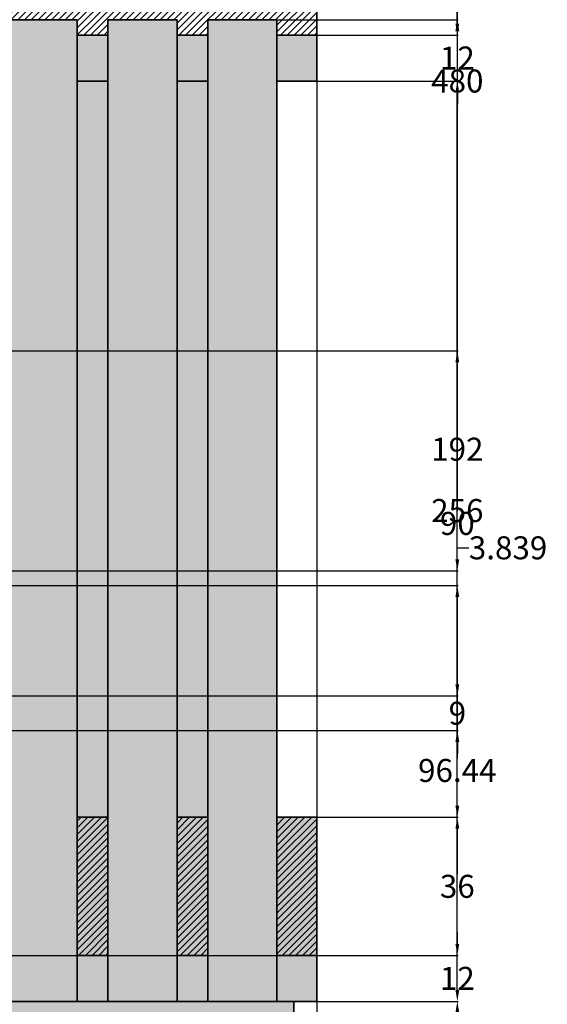
# Model space of a CAD drawing. Units: inches. Extents: x 126 to 726, y 86 to 888.
# Tile 11 of 13: x 589 to 726, y 354 to 611. Entities that reach past the tile are written whole.
import ezdxf

# ---------------------------------------------------------------- set-up
doc = ezdxf.new("R2010")
doc.units = ezdxf.units.IN
doc.header["$MEASUREMENT"] = 0
for name, color, linetype, lineweight in [('A-ANNO-DIMS', 2, 'Continuous', 18), ('A-ELEV', 7, 'Continuous', 35), ('A-ELEV-PATT', 8, 'Continuous', 13)]:
    doc.layers.add(name, color=color, linetype=linetype, lineweight=lineweight)
doc.styles.get("Standard").update_dxf_attribs({"font": 'arial.ttf'})
doc.dimstyles.get("Standard").update_dxf_attribs({"dimtxt": 6, "dimasz": 3, "dimexe": 0.18, "dimexo": 0.0625, "dimgap": 0.09, "dimtad": 0, "dimtih": 1, "dimtoh": 1, "dimdec": 0, "dimzin": 0, "dimdsep": 46, "dimlunit": 3, "dimtxsty": 'Standard', "dimcen": 0.09, "dimadec": 0, "dimazin": 0, "dimtfac": 1, "dimtdec": 0, "dimtofl": 0, "dimtmove": 0, "dimatfit": 3, "dimfxl": 1, "dimtolj": 1, "dimtzin": 0, "dimarcsym": 0})

# ---------------------------------------------------------------- blocks, each defined once
blk = doc.blocks.new('*D13')
at = {"layer": 'A-ANNO-DIMS', "color": 0, "lineweight": -2, "transparency": 16777216}
for p, q in [((665.97, 642.98), (665.97, 90.21)), ((185.97, 126.98), (185.97, 90.21)), ((188.97, 90.39), (419.15, 90.39)), ((662.97, 90.39), (432.8, 90.39))]:
    blk.add_line(p, q, dxfattribs=at)
at = {"layer": 'A-ANNO-DIMS', "color": 0, "transparency": 16777216}
for points in [[(188.97, 90.89), (188.97, 89.89), (185.97, 90.39)], [(662.97, 90.89), (662.97, 89.89), (665.97, 90.39)]]:
    blk.add_solid(points, dxfattribs=at)
at = {"layer": 'Defpoints', "color": 0, "transparency": 16777216}
for p in [(665.97, 643.04), (185.97, 127.04), (665.97, 90.39)]:
    blk.add_point(p, dxfattribs=at)
at = {"layer": 'A-ANNO-DIMS', "color": 0, "transparency": 16777216, "insert": (425.97, 90.39), "char_height": 6, "attachment_point": 5}
blk.add_mtext('\\A1;480', dxfattribs=at)
blk = doc.blocks.new('*D28')
at = {"layer": 'A-ANNO-DIMS', "color": 0, "lineweight": -2, "transparency": 16777216}
for p, q in [((666.04, 355.04), (702.8, 355.04)), ((702.62, 352.04), (702.62, 244.2)), ((702.62, 130.04), (702.62, 237.89)), ((660.11, 127.04), (702.8, 127.04))]:
    blk.add_line(p, q, dxfattribs=at)
at = {"layer": 'A-ANNO-DIMS', "color": 0, "transparency": 16777216}
for points in [[(702.12, 352.04), (703.12, 352.04), (702.62, 355.04)], [(702.12, 130.04), (703.12, 130.04), (702.62, 127.04)]]:
    blk.add_solid(points, dxfattribs=at)
at = {"layer": 'Defpoints', "color": 0, "transparency": 16777216}
for p in [(665.97, 355.04), (702.62, 355.04), (660.05, 127.04)]:
    blk.add_point(p, dxfattribs=at)
at = {"layer": 'A-ANNO-DIMS', "color": 0, "transparency": 16777216, "insert": (702.62, 241.04), "char_height": 6, "attachment_point": 5}
blk.add_mtext('\\A1;228', dxfattribs=at)
blk = doc.blocks.new('*D29')
at = {"layer": 'A-ANNO-DIMS', "color": 0, "lineweight": -2, "transparency": 16777216}
for p, q in [((606.04, 835.04), (702.8, 835.04)), ((702.62, 832.04), (702.62, 598.2)), ((702.62, 358.04), (702.62, 591.89)), ((666.04, 355.04), (702.8, 355.04))]:
    blk.add_line(p, q, dxfattribs=at)
at = {"layer": 'A-ANNO-DIMS', "color": 0, "transparency": 16777216}
for points in [[(702.12, 832.04), (703.12, 832.04), (702.62, 835.04)], [(702.12, 358.04), (703.12, 358.04), (702.62, 355.04)]]:
    blk.add_solid(points, dxfattribs=at)
at = {"layer": 'Defpoints', "color": 0, "transparency": 16777216}
for p in [(605.97, 835.04), (702.62, 835.04), (665.97, 355.04)]:
    blk.add_point(p, dxfattribs=at)
at = {"layer": 'A-ANNO-DIMS', "color": 0, "transparency": 16777216, "insert": (702.62, 595.04), "char_height": 6, "attachment_point": 5}
blk.add_mtext('\\A1;480', dxfattribs=at)
blk = doc.blocks.new('*D34')
at = {"layer": 'A-ANNO-DIMS', "color": 0, "lineweight": -2, "transparency": 16777216}
for p, q in [((362.73, 524.68), (702.8, 524.68)), ((702.62, 521.68), (702.62, 482.84)), ((702.62, 437.68), (702.62, 476.53)), ((362.73, 434.68), (702.8, 434.68))]:
    blk.add_line(p, q, dxfattribs=at)
at = {"layer": 'A-ANNO-DIMS', "color": 0, "transparency": 16777216}
for points in [[(702.12, 521.68), (703.12, 521.68), (702.62, 524.68)], [(702.12, 437.68), (703.12, 437.68), (702.62, 434.68)]]:
    blk.add_solid(points, dxfattribs=at)
at = {"layer": 'Defpoints', "color": 0, "transparency": 16777216}
for p in [(362.67, 524.68), (702.62, 524.68), (362.67, 434.68)]:
    blk.add_point(p, dxfattribs=at)
at = {"layer": 'A-ANNO-DIMS', "color": 0, "transparency": 16777216, "insert": (702.62, 479.68), "char_height": 6, "attachment_point": 5}
blk.add_mtext('\\A1;90', dxfattribs=at)
blk = doc.blocks.new('*D35')
at = {"layer": 'A-ANNO-DIMS', "color": 0, "lineweight": -2, "transparency": 16777216}
for p, q in [((702.624909, 437.684516), (702.624909, 440.684516)), ((362.728342, 434.684516), (702.804909, 434.684516)), ((371.728342, 425.684516), (702.804909, 425.684516)), ((702.624909, 422.684516), (702.624909, 419.684516))]:
    blk.add_line(p, q, dxfattribs=at)
at = {"layer": 'A-ANNO-DIMS', "color": 0, "transparency": 16777216}
for points in [[(702.124909, 437.684516), (703.124909, 437.684516), (702.624909, 434.684516)], [(702.124909, 422.684516), (703.124909, 422.684516), (702.624909, 425.684516)]]:
    blk.add_solid(points, dxfattribs=at)
at = {"layer": 'Defpoints', "color": 0, "transparency": 16777216}
for p in [(362.665842, 434.684516), (702.624909, 434.684516), (371.665842, 425.684516)]:
    blk.add_point(p, dxfattribs=at)
at = {"layer": 'A-ANNO-DIMS', "color": 0, "transparency": 16777216, "insert": (702.624909, 430.184516), "char_height": 6, "attachment_point": 5}
blk.add_mtext('\\A1;9', dxfattribs=at)
blk = doc.blocks.new('*D41')
at = {"layer": 'A-ANNO-DIMS', "color": 0, "lineweight": -2, "transparency": 16777216}
for p, q in [((429.97, 607.1), (429.97, 883.87)), ((432.97, 883.69), (541.21, 883.69)), ((662.97, 883.69), (554.74, 883.69)), ((665.97, 607.1), (665.97, 883.87))]:
    blk.add_line(p, q, dxfattribs=at)
at = {"layer": 'A-ANNO-DIMS', "color": 0, "transparency": 16777216}
for points in [[(432.97, 884.19), (432.97, 883.19), (429.97, 883.69)], [(662.97, 884.19), (662.97, 883.19), (665.97, 883.69)]]:
    blk.add_solid(points, dxfattribs=at)
at = {"layer": 'Defpoints', "color": 0, "transparency": 16777216}
for p in [(665.97, 883.69), (429.97, 607.04), (665.97, 607.04)]:
    blk.add_point(p, dxfattribs=at)
at = {"layer": 'A-ANNO-DIMS', "color": 0, "transparency": 16777216, "insert": (547.97, 883.69), "char_height": 6, "attachment_point": 5}
blk.add_mtext('\\A1;236', dxfattribs=at)
blk = doc.blocks.new('*D42')
at = {"layer": 'A-ANNO-DIMS', "color": 0, "lineweight": -2, "transparency": 16777216}
for p, q in [((429.97, 354.98), (429.97, 90.21)), ((665.97, 354.98), (665.97, 90.21)), ((432.97, 90.39), (541.21, 90.39)), ((662.97, 90.39), (554.74, 90.39))]:
    blk.add_line(p, q, dxfattribs=at)
at = {"layer": 'A-ANNO-DIMS', "color": 0, "transparency": 16777216}
for points in [[(432.97, 90.89), (432.97, 89.89), (429.97, 90.39)], [(662.97, 90.89), (662.97, 89.89), (665.97, 90.39)]]:
    blk.add_solid(points, dxfattribs=at)
at = {"layer": 'Defpoints', "color": 0, "transparency": 16777216}
for p in [(429.97, 355.04), (665.97, 355.04), (665.97, 90.39)]:
    blk.add_point(p, dxfattribs=at)
at = {"layer": 'A-ANNO-DIMS', "color": 0, "transparency": 16777216, "insert": (547.97, 90.39), "char_height": 6, "attachment_point": 5}
blk.add_mtext('\\A1;236', dxfattribs=at)
blk = doc.blocks.new('*D45')
at = {"layer": 'A-ANNO-DIMS', "color": 0, "lineweight": -2, "transparency": 16777216}
for p, q in [((702.624909, 370.042369), (702.624909, 373.042369)), ((666.037409, 367.042369), (702.804909, 367.042369)), ((666.037409, 355.042369), (702.804909, 355.042369)), ((702.624909, 352.042369), (702.624909, 349.042369))]:
    blk.add_line(p, q, dxfattribs=at)
at = {"layer": 'A-ANNO-DIMS', "color": 0, "transparency": 16777216}
for points in [[(702.124909, 370.042369), (703.124909, 370.042369), (702.624909, 367.042369)], [(702.124909, 352.042369), (703.124909, 352.042369), (702.624909, 355.042369)]]:
    blk.add_solid(points, dxfattribs=at)
at = {"layer": 'Defpoints', "color": 0, "transparency": 16777216}
for p in [(665.974909, 367.042369), (702.624909, 367.042369), (665.974909, 355.042369)]:
    blk.add_point(p, dxfattribs=at)
at = {"layer": 'A-ANNO-DIMS', "color": 0, "transparency": 16777216, "insert": (702.624909, 361.042369), "char_height": 6, "attachment_point": 5}
blk.add_mtext('\\A1;12', dxfattribs=at)
blk = doc.blocks.new('*D46')
at = {"layer": 'A-ANNO-DIMS', "color": 0, "lineweight": -2, "transparency": 16777216}
for p, q in [((666.04, 403.04), (702.8, 403.04)), ((702.62, 400.04), (702.62, 388.2)), ((702.62, 370.04), (702.62, 381.89)), ((666.04, 367.04), (702.8, 367.04))]:
    blk.add_line(p, q, dxfattribs=at)
at = {"layer": 'A-ANNO-DIMS', "color": 0, "transparency": 16777216}
for points in [[(702.12, 400.04), (703.12, 400.04), (702.62, 403.04)], [(702.12, 370.04), (703.12, 370.04), (702.62, 367.04)]]:
    blk.add_solid(points, dxfattribs=at)
at = {"layer": 'Defpoints', "color": 0, "transparency": 16777216}
for p in [(665.97, 403.04), (702.62, 403.04), (665.97, 367.04)]:
    blk.add_point(p, dxfattribs=at)
at = {"layer": 'A-ANNO-DIMS', "color": 0, "transparency": 16777216, "insert": (702.62, 385.04), "char_height": 6, "attachment_point": 5}
blk.add_mtext('\\A1;36', dxfattribs=at)
blk = doc.blocks.new('*D47')
at = {"layer": 'A-ANNO-DIMS', "color": 0, "lineweight": -2, "transparency": 16777216}
for p, q in [((666.04, 595.04), (702.8, 595.04)), ((702.62, 592.04), (702.62, 502.2)), ((702.62, 406.04), (702.62, 495.89)), ((666.04, 403.04), (702.8, 403.04))]:
    blk.add_line(p, q, dxfattribs=at)
at = {"layer": 'A-ANNO-DIMS', "color": 0, "transparency": 16777216}
for points in [[(702.12, 592.04), (703.12, 592.04), (702.62, 595.04)], [(702.12, 406.04), (703.12, 406.04), (702.62, 403.04)]]:
    blk.add_solid(points, dxfattribs=at)
at = {"layer": 'Defpoints', "color": 0, "transparency": 16777216}
for p in [(665.97, 595.04), (702.62, 595.04), (665.97, 403.04)]:
    blk.add_point(p, dxfattribs=at)
at = {"layer": 'A-ANNO-DIMS', "color": 0, "transparency": 16777216, "insert": (702.62, 499.04), "char_height": 6, "attachment_point": 5}
blk.add_mtext('\\A1;192', dxfattribs=at)
blk = doc.blocks.new('*D48')
at = {"layer": 'A-ANNO-DIMS', "color": 0, "lineweight": -2, "transparency": 16777216}
for p, q in [((702.624909, 610.042369), (702.624909, 613.042369)), ((666.037409, 607.042369), (702.804909, 607.042369)), ((666.037409, 595.042369), (702.804909, 595.042369)), ((702.624909, 592.042369), (702.624909, 589.042369))]:
    blk.add_line(p, q, dxfattribs=at)
at = {"layer": 'A-ANNO-DIMS', "color": 0, "transparency": 16777216}
for points in [[(702.124909, 610.042369), (703.124909, 610.042369), (702.624909, 607.042369)], [(702.124909, 592.042369), (703.124909, 592.042369), (702.624909, 595.042369)]]:
    blk.add_solid(points, dxfattribs=at)
at = {"layer": 'Defpoints', "color": 0, "transparency": 16777216}
for p in [(665.974909, 607.042369), (702.624909, 607.042369), (665.974909, 595.042369)]:
    blk.add_point(p, dxfattribs=at)
at = {"layer": 'A-ANNO-DIMS', "color": 0, "transparency": 16777216, "insert": (702.624909, 601.042369), "char_height": 6, "attachment_point": 5}
blk.add_mtext('\\A1;12', dxfattribs=at)
blk = doc.blocks.new('*D49')
at = {"layer": 'A-ANNO-DIMS', "color": 0, "lineweight": -2, "transparency": 16777216}
for p, q in [((666.04, 643.04), (702.8, 643.04)), ((702.62, 640.04), (702.62, 628.2)), ((702.62, 610.04), (702.62, 621.89)), ((666.04, 607.04), (702.8, 607.04))]:
    blk.add_line(p, q, dxfattribs=at)
at = {"layer": 'A-ANNO-DIMS', "color": 0, "transparency": 16777216}
for points in [[(702.12, 640.04), (703.12, 640.04), (702.62, 643.04)], [(702.12, 610.04), (703.12, 610.04), (702.62, 607.04)]]:
    blk.add_solid(points, dxfattribs=at)
at = {"layer": 'Defpoints', "color": 0, "transparency": 16777216}
for p in [(665.97, 643.04), (702.62, 643.04), (665.97, 607.04)]:
    blk.add_point(p, dxfattribs=at)
at = {"layer": 'A-ANNO-DIMS', "color": 0, "transparency": 16777216, "insert": (702.62, 625.04), "char_height": 6, "attachment_point": 5}
blk.add_mtext('\\A1;36', dxfattribs=at)
blk = doc.blocks.new('*D57')
at = {"layer": 'A-ANNO-DIMS', "color": 0, "lineweight": -2, "transparency": 16777216}
for p, q in [((655.64, 611.04), (702.8, 611.04)), ((702.62, 608.04), (702.62, 486.2)), ((702.62, 358.04), (702.62, 479.89)), ((655.64, 355.04), (702.8, 355.04))]:
    blk.add_line(p, q, dxfattribs=at)
at = {"layer": 'A-ANNO-DIMS', "color": 0, "transparency": 16777216}
for points in [[(702.12, 608.04), (703.12, 608.04), (702.62, 611.04)], [(702.12, 358.04), (703.12, 358.04), (702.62, 355.04)]]:
    blk.add_solid(points, dxfattribs=at)
at = {"layer": 'Defpoints', "color": 0, "transparency": 16777216}
for p in [(655.58, 611.04), (702.62, 611.04), (655.58, 355.04)]:
    blk.add_point(p, dxfattribs=at)
at = {"layer": 'A-ANNO-DIMS', "color": 0, "transparency": 16777216, "insert": (702.62, 483.04), "char_height": 6, "attachment_point": 5}
blk.add_mtext('\\A1;256', dxfattribs=at)
blk = doc.blocks.new('*D62')
at = {"layer": 'A-ANNO-DIMS', "color": 0, "lineweight": -2, "transparency": 16777216}
for p, q in [((702.62, 470.32), (702.62, 473.32)), ((702.62, 473.32), (705.62, 473.32)), ((515.5, 467.32), (702.8, 467.32)), ((515.5, 463.48), (702.8, 463.48)), ((702.62, 460.48), (702.62, 457.48))]:
    blk.add_line(p, q, dxfattribs=at)
at = {"layer": 'A-ANNO-DIMS', "color": 0, "transparency": 16777216}
for points in [[(702.12, 470.32), (703.12, 470.32), (702.62, 467.32)], [(702.12, 460.48), (703.12, 460.48), (702.62, 463.48)]]:
    blk.add_solid(points, dxfattribs=at)
at = {"layer": 'Defpoints', "color": 0, "transparency": 16777216}
for p in [(515.44, 467.32), (702.62, 467.32), (515.44, 463.48)]:
    blk.add_point(p, dxfattribs=at)
at = {"layer": 'A-ANNO-DIMS', "color": 0, "transparency": 16777216, "insert": (715.84, 473.32), "char_height": 6, "attachment_point": 5}
blk.add_mtext('\\A1;3.839', dxfattribs=at)
blk = doc.blocks.new('*D64')
at = {"layer": 'A-ANNO-DIMS', "color": 0, "lineweight": -2, "transparency": 16777216}
for p, q in [((501.88, 463.48), (702.8, 463.48)), ((702.62, 460.48), (702.62, 418.42)), ((702.62, 370.04), (702.62, 412.11)), ((486.04, 367.04), (702.8, 367.04))]:
    blk.add_line(p, q, dxfattribs=at)
at = {"layer": 'A-ANNO-DIMS', "color": 0, "transparency": 16777216}
for points in [[(702.12, 460.48), (703.12, 460.48), (702.62, 463.48)], [(702.12, 370.04), (703.12, 370.04), (702.62, 367.04)]]:
    blk.add_solid(points, dxfattribs=at)
at = {"layer": 'Defpoints', "color": 0, "transparency": 16777216}
for p in [(501.82, 463.48), (485.97, 367.04), (702.62, 367.04)]:
    blk.add_point(p, dxfattribs=at)
at = {"layer": 'A-ANNO-DIMS', "color": 0, "transparency": 16777216, "insert": (702.62, 415.26), "char_height": 6, "attachment_point": 5}
blk.add_mtext('\\A1;96.44', dxfattribs=at)

msp = doc.modelspace()

# ---------------------------------------------------------------- hatches: boundary and pattern name
at = {"layer": 'A-ELEV-PATT'}
h = msp.add_hatch(dxfattribs=at)
h.set_pattern_fill('ANSI31', color=256, scale=10)
h.paths.add_polyline_path([(585.5818, 607.0424), (585.5818, 611.0424), (603.5818, 611.0424), (603.5818, 607.0424), (611.5818, 607.0424), (611.5818, 611.0424), (629.5818, 611.0424), (629.5818, 607.0424), (637.5818, 607.0424), (637.5818, 611.0424), (655.5818, 611.0424), (655.5818, 607.0424), (665.9749, 607.0424), (665.9749, 643.0424), (485.9749, 643.0424), (485.9749, 607.0424)])
h = msp.add_hatch(color=256, dxfattribs=at)
h.dxf.hatch_style = 1
h.paths.add_polyline_path([(655.5818, 607.0424), (655.5818, 611.0424), (637.5818, 611.0424), (637.5818, 355.0424), (655.5818, 355.0424)])
h.paths.add_polyline_path([(629.5818, 611.0424), (611.5818, 611.0424), (611.5818, 355.0424), (629.5818, 355.0424)])
h.paths.add_polyline_path([(585.5818, 355.0424), (603.5818, 355.0424), (603.5818, 611.0424), (585.5818, 611.0424), (585.5818, 607.0424)])
h = msp.add_hatch(color=256, dxfattribs=at)
h.dxf.hatch_style = 1
h.paths.add_polyline_path([(611.5818, 367.0424), (603.5818, 367.0424), (603.5818, 355.0424), (611.5818, 355.0424)])
h.paths.add_polyline_path([(637.5818, 355.0424), (637.5818, 367.0424), (629.5818, 367.0424), (629.5818, 355.0424)])
h.paths.add_polyline_path([(665.9749, 355.0424), (665.9749, 367.0424), (655.5818, 367.0424), (655.5818, 355.0424)])
h.paths.add_polyline_path([(665.9749, 607.0424), (655.5818, 607.0424), (655.5818, 595.0424), (665.9749, 595.0424)])
h.paths.add_polyline_path([(629.5818, 595.0424), (637.5818, 595.0424), (637.5818, 607.0424), (629.5818, 607.0424)])
h.paths.add_polyline_path([(603.5818, 595.0424), (611.5818, 595.0424), (611.5818, 607.0424), (603.5818, 607.0424)])
h = msp.add_hatch(color=256, dxfattribs=at)
h.dxf.hatch_style = 1
h.paths.add_polyline_path([(485.9749, 595.0424), (485.9749, 564.6845), (585.5818, 564.6845), (585.5818, 595.0424)])
h.paths.add_polyline_path([(660.0469, 325.0424), (660.0469, 355.0424), (485.9749, 355.0424), (485.9749, 325.0424)])
h = msp.add_hatch(color=256, dxfattribs=at)
h.dxf.hatch_style = 1
h.paths.add_polyline_path([(611.5818, 595.0424), (603.5818, 595.0424), (603.5818, 403.0424), (611.5818, 403.0424)])
h.paths.add_polyline_path([(637.5818, 595.0424), (629.5818, 595.0424), (629.5818, 403.0424), (637.5818, 403.0424)])
h = msp.add_hatch(color=256, dxfattribs=at)
h.dxf.hatch_style = 1
h.paths.add_polyline_path([(611.5818, 403.0424), (603.5818, 403.0424), (603.5818, 367.0424), (611.5818, 367.0424)])
h.paths.add_polyline_path([(637.5818, 403.0424), (629.5818, 403.0424), (629.5818, 367.0424), (637.5818, 367.0424)])
h.paths.add_polyline_path([(665.9749, 403.0424), (655.5818, 403.0424), (655.5818, 367.0424), (665.9749, 367.0424)])
h = msp.add_hatch(dxfattribs=at)
h.set_pattern_fill('ANSI31', color=256, scale=10)
h.paths.add_polyline_path([(611.5818, 403.0424), (603.5818, 403.0424), (603.5818, 367.0424), (611.5818, 367.0424)])
h.paths.add_polyline_path([(637.5818, 403.0424), (629.5818, 403.0424), (629.5818, 367.0424), (637.5818, 367.0424)])
h.paths.add_polyline_path([(665.9749, 403.0424), (655.5818, 403.0424), (655.5818, 367.0424), (665.9749, 367.0424)])

# ---------------------------------------------------------------- linework, layer by layer
at = {"layer": 'A-ELEV'}
for p, q in [((665.9749, 595.0424), (665.9749, 643.0424)), ((603.5818, 611.0424), (585.5818, 611.0424)), ((603.5818, 355.0424), (603.5818, 611.0424)), ((611.5818, 355.0424), (611.5818, 611.0424)), ((629.5818, 611.0424), (611.5818, 611.0424)), ((629.5818, 355.0424), (629.5818, 611.0424)), ((637.5818, 355.0424), (637.5818, 611.0424)), ((655.5818, 611.0424), (637.5818, 611.0424)), ((655.5818, 611.0424), (655.5818, 607.0424)), ((603.5818, 607.0424), (611.5818, 607.0424)), ((629.5818, 607.0424), (637.5818, 607.0424)), ((655.5818, 355.0424), (655.5818, 607.0424)), ((655.5818, 607.0424), (665.9749, 607.0424)), ((611.5818, 595.0424), (603.5818, 595.0424)), ((637.5818, 595.0424), (629.5818, 595.0424)), ((665.9749, 595.0424), (655.5818, 595.0424)), ((603.5818, 403.0424), (611.5818, 403.0424)), ((629.5818, 403.0424), (637.5818, 403.0424)), ((655.5818, 403.0424), (665.9749, 403.0424)), ((665.9749, 355.0424), (665.9749, 403.0424)), ((603.5818, 367.0424), (611.5818, 367.0424)), ((629.5818, 367.0424), (637.5818, 367.0424)), ((655.5818, 367.0424), (665.9749, 367.0424)), ((665.9749, 355.0424), (437.9749, 355.0424)), ((660.0469, 355.0424), (660.0469, 127.0424))]:
    msp.add_line(p, q, dxfattribs=at)

# ---------------------------------------------------------------- dimensions: what is measured, and where the dimension line sits
at = {"layer": 'A-ANNO-DIMS'}
for base, p1, p2, picture, middle in [((665.9749, 883.6924), (429.9749, 607.0424), (665.9749, 607.0424), '*D41', (547.9749, 883.6924)), ((665.9749, 90.3924), (185.9749, 127.0424), (665.9749, 643.0424), '*D13', (425.9749, 90.3924)), ((665.9749, 90.3924), (429.9749, 355.0424), (665.9749, 355.0424), '*D42', (547.9749, 90.3924))]:
    dim = msp.add_linear_dim(base=base, p1=p1, p2=p2, dimstyle='Standard', override={"dimdec": 0, "dimlfac": 1, "dimrnd": 0, "dimzin": 0, "dimdsep": 46, "dimlunit": 2}, dxfattribs=at)
    dim.commit()
    dim.dimension.update_dxf_attribs({"geometry": picture, "text_midpoint": middle})
for base, p1, p2, override, picture, middle in [((702.6249, 835.0424), (665.9749, 355.0424), (605.9749, 835.0424), {"dimdec": 0, "dimlfac": 1, "dimrnd": 0, "dimzin": 0, "dimdsep": 46, "dimlunit": 2}, '*D29', (702.6249, 595.0424)), ((702.6249, 643.0424), (665.9749, 607.0424), (665.9749, 643.0424), {"dimdec": 0, "dimlfac": 1, "dimrnd": 0, "dimzin": 0, "dimdsep": 46, "dimlunit": 2}, '*D49', (702.6249, 625.0424)), ((702.6249, 607.0424), (665.9749, 595.0424), (665.9749, 607.0424), {"dimdec": 0, "dimlfac": 1, "dimrnd": 0, "dimzin": 0, "dimdsep": 46, "dimlunit": 2}, '*D48', (702.6249, 601.0424)), ((702.6249, 611.0424), (655.5818, 355.0424), (655.5818, 611.0424), {"dimdec": 0, "dimlfac": 1, "dimrnd": 0, "dimzin": 0, "dimdsep": 46, "dimlunit": 2}, '*D57', (702.6249, 483.0424)), ((702.6249, 595.0424), (665.9749, 403.0424), (665.9749, 595.0424), {"dimdec": 0, "dimlfac": 1, "dimrnd": 0, "dimzin": 0, "dimdsep": 46, "dimlunit": 2}, '*D47', (702.6249, 499.0424)), ((702.6249, 524.6845), (362.6658, 434.6845), (362.6658, 524.6845), {"dimdec": 0, "dimlfac": 1, "dimrnd": 0, "dimzin": 0, "dimdsep": 46, "dimlunit": 2}, '*D34', (702.6249, 479.6845)), ((702.6249, 467.321), (515.4403, 463.4817), (515.4403, 467.321), {"dimdec": 3, "dimlfac": 1, "dimrnd": 0, "dimzin": 0, "dimdsep": 46, "dimlunit": 2}, '*D62', (715.8425, 473.321)), ((702.6249, 367.0424), (501.8163, 463.4817), (485.9749, 367.0424), {"dimdec": 2, "dimlfac": 1, "dimrnd": 0, "dimzin": 0, "dimdsep": 46, "dimlunit": 2}, '*D64', (702.6249, 415.262)), ((702.6249, 434.6845), (371.6658, 425.6845), (362.6658, 434.6845), {"dimdec": 0, "dimlfac": 1, "dimrnd": 0, "dimzin": 0, "dimdsep": 46, "dimlunit": 2}, '*D35', (702.6249, 430.1845)), ((702.6249, 403.0424), (665.9749, 367.0424), (665.9749, 403.0424), {"dimdec": 0, "dimlfac": 1, "dimrnd": 0, "dimzin": 0, "dimdsep": 46, "dimlunit": 2}, '*D46', (702.6249, 385.0424)), ((702.6249, 367.0424), (665.9749, 355.0424), (665.9749, 367.0424), {"dimdec": 0, "dimlfac": 1, "dimrnd": 0, "dimzin": 0, "dimdsep": 46, "dimlunit": 2}, '*D45', (702.6249, 361.0424)), ((702.6249, 355.0424), (660.0469, 127.0424), (665.9749, 355.0424), {"dimdec": 0, "dimlfac": 1, "dimrnd": 0, "dimzin": 0, "dimdsep": 46, "dimlunit": 2}, '*D28', (702.6249, 241.0424))]:
    dim = msp.add_linear_dim(base=base, p1=p1, p2=p2, angle=90, dimstyle='Standard', override=override, dxfattribs=at)
    dim.commit()
    dim.dimension.update_dxf_attribs({"geometry": picture, "text_midpoint": middle})

doc.saveas('drawing.dxf')
